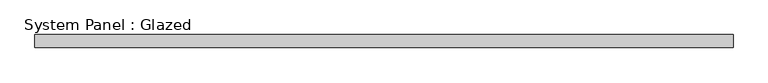
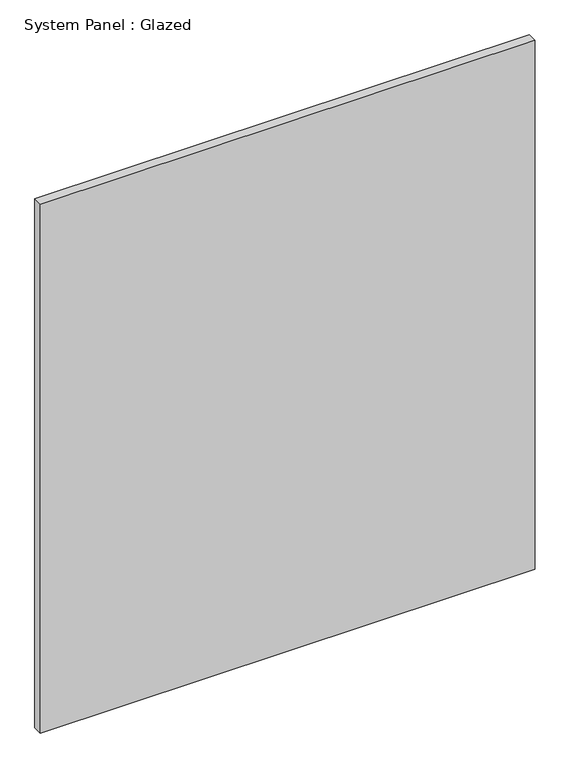
"""IFC4 building model written with IfcOpenShell, lengths in millimetres: plate geometry, System Panel : Glazed."""

from ifc_helpers import new_model, si_unit, origin, origin_with_axes, place, context, project, spatial, polyline, outline, extrude, source, transform, mapped, element, save


def system_panel_glazed_616dcef8(model_context):
    return source(origin(), model_context, "Body", "SweptSolid", [
        extrude(outline(polyline([(679.45, 19.05), (-679.45, 19.05), (-679.45, 44.45), (679.45, 44.45), (679.45, 19.05)])), origin_with_axes(), (0.0, 0.0, 1.0), 1535.7829369),
    ])


if __name__ == "__main__":
    model = new_model("IFC4")
    model_context = context("Model", 3, world=origin())
    ifc_project = project(units=[si_unit("LENGTHUNIT", "METRE", prefix="MILLI")], contexts=[model_context])
    site = spatial("IfcSite", under=ifc_project)
    building = spatial("IfcBuilding", under=site)
    placement = place(None, origin())
    system_panel_glazed_shape = system_panel_glazed_616dcef8(model_context)
    element("IfcPlate", 1, ObjectType="System Panel : Glazed", at=placement, inside=building, context=model_context, shape_type="MappedRepresentation", body=[
        mapped(system_panel_glazed_shape, transform((0.0, 0.0, 0.0), x_axis=(1.0, 0.0, 0.0), y_axis=(0.0, 1.0, 0.0), z_axis=(0.0, 0.0, 1.0))),
    ])
    save(model, "model.ifc")

# Revit data of these elements
# Type "System Panel : Glazed"
#   Construction Type Id = "GSP4R"
#   Analytic Construction = "1/8 in Pilkington single glazing"
#   Visual Light Transmittance = 0.9
#   Solar Heat Gain Coefficient = 0.86
#   Heat Transfer Coefficient (U) = 1.18115 BTU/(h·ft²·°F)
#   Define Thermal Properties by = 1
# Element 1 (IfcPlate, "System Panel : Glazed")
#   Materials on its faces: "Glass"
# Materials
#   "Glass": class "Glass", colour RGB 0 128 192, transparency 0.75, Description = "Soda Lime Glass", Cost = 0
